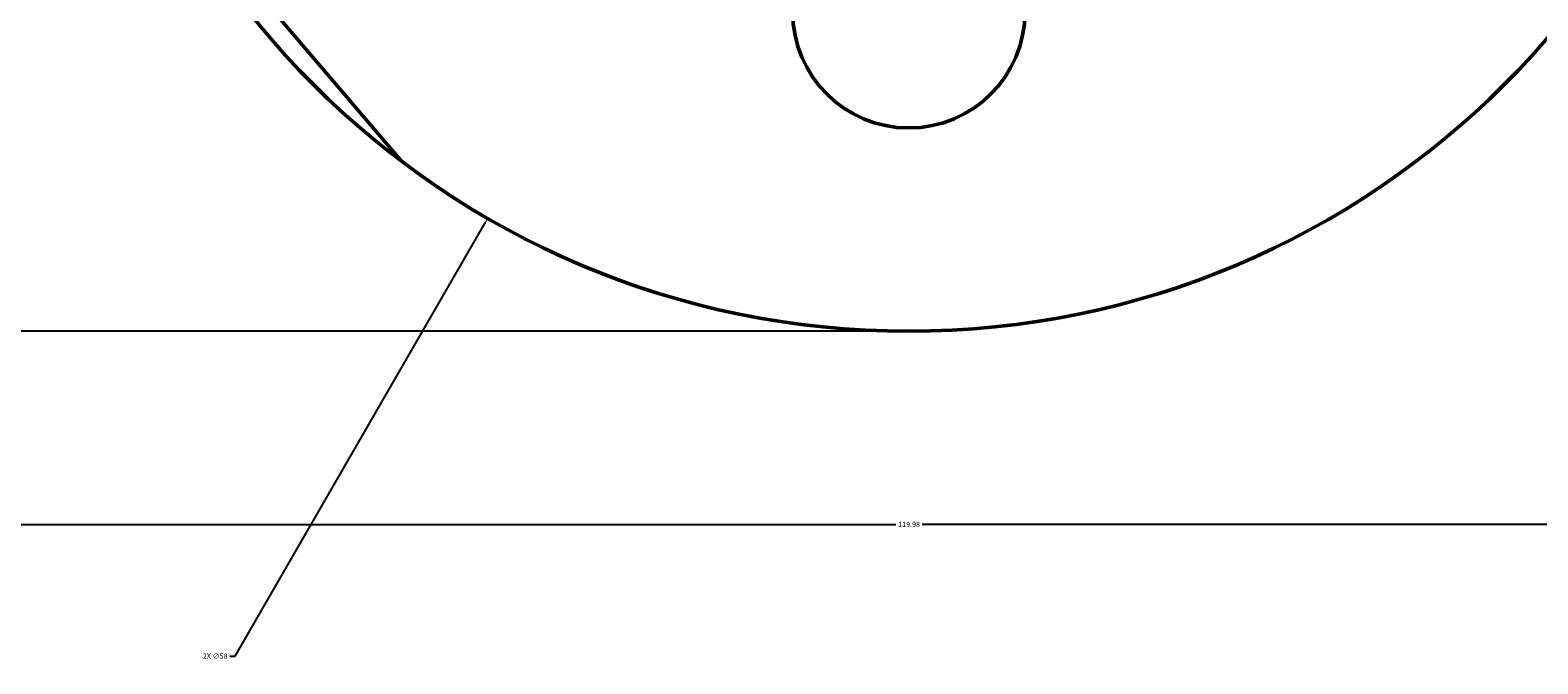
# Model space of a CAD drawing. Units: inches. Extents: x -11 to 126, y -62 to 82.
# Tile 2 of 10: x 29 to 81, y -62 to -40. Entities that reach past the tile are written whole.
import ezdxf

# ---------------------------------------------------------------- set-up
doc = ezdxf.new("R2010")
doc.units = ezdxf.units.IN
doc.header["$MEASUREMENT"] = 0
doc.layers.add('M-DIMS', color=2, linetype='Continuous', lineweight=18)
doc.layers.add('M-OUTL', color=7, linetype='Continuous', lineweight=50)
doc.styles.get("Standard").update_dxf_attribs({"font": 'arial.ttf'})
doc.dimstyles.get("Standard").update_dxf_attribs({"dimtxt": 0.18, "dimasz": 0.18, "dimexe": 0.18, "dimexo": 0.0625, "dimgap": 0.09, "dimtad": 0, "dimtih": 1, "dimtoh": 1, "dimdec": 4, "dimzin": 0, "dimdsep": 46, "dimtxsty": 'Standard', "dimcen": 0.09, "dimadec": 0, "dimazin": 0, "dimtfac": 1, "dimtdec": 4, "dimtofl": 0, "dimtmove": 0, "dimatfit": 3, "dimfxl": 1, "dimtolj": 1, "dimtzin": 0, "dimarcsym": 0})

# ---------------------------------------------------------------- blocks, each defined once
blk = doc.blocks.new('*U3')
blk.add_circle((0, 0), 4)
blk = doc.blocks.new('*U4')
at = {"layer": 'M-OUTL', "color": 0, "linetype": 'ByBlock', "lineweight": -2, "transparency": 16777216}
blk.add_blockref('*U3', (59.232, -3.646), dxfattribs=at)
for p, rotation in [((43.643, -12.646), 59.99999999999999), ((74.82, -12.646), 300), ((43.643, -30.646), 120), ((74.82, -30.646), 240), ((59.232, -39.646), 180)]:
    blk.add_blockref('*U3', p, dxfattribs=dict(at, rotation=rotation))
blk = doc.blocks.new('*D5')
at = {"layer": 'Defpoints', "color": 0, "transparency": 16777216}
for p in [(119.232, 12.354), (-0.749, 11.479), (119.232, -57.296)]:
    blk.add_point(p, dxfattribs=at)
at = {"layer": 'M-DIMS', "color": 0, "lineweight": -2, "transparency": 16777216}
for p, q in [((119.232, 12.292), (119.232, -57.476)), ((-0.749, 11.416), (-0.749, -57.476)), ((-0.569, -57.296), (58.786, -57.296)), ((119.052, -57.296), (59.696, -57.296))]:
    blk.add_line(p, q, dxfattribs=at)
at = {"layer": 'M-DIMS', "color": 0, "transparency": 16777216}
for points in [[(-0.569, -57.266), (-0.569, -57.326), (-0.749, -57.296)], [(119.052, -57.266), (119.052, -57.326), (119.232, -57.296)]]:
    blk.add_solid(points, dxfattribs=at)
at = {"layer": 'M-DIMS', "color": 0, "transparency": 16777216, "insert": (59.241, -57.296), "char_height": 0.18, "attachment_point": 5}
blk.add_mtext('\\A1;119.98', dxfattribs=at)
blk = doc.blocks.new('*D6')
at = {"layer": 'Defpoints', "color": 0, "transparency": 16777216}
for p in [(-7.399, 75.354), (59.232, 75.354), (59.232, -50.646)]:
    blk.add_point(p, dxfattribs=at)
at = {"layer": 'M-DIMS', "color": 0, "lineweight": -2, "transparency": 16777216}
for p, q in [((59.169, 75.354), (-7.579, 75.354)), ((-7.399, 75.174), (-7.399, 12.536)), ((-7.399, -50.466), (-7.399, 12.172)), ((59.169, -50.646), (-7.579, -50.646))]:
    blk.add_line(p, q, dxfattribs=at)
at = {"layer": 'M-DIMS', "color": 0, "transparency": 16777216}
for points in [[(-7.429, 75.174), (-7.369, 75.174), (-7.399, 75.354)], [(-7.429, -50.466), (-7.369, -50.466), (-7.399, -50.646)]]:
    blk.add_solid(points, dxfattribs=at)
at = {"layer": 'M-DIMS', "color": 0, "transparency": 16777216, "insert": (-7.399, 12.354), "char_height": 0.18, "attachment_point": 5}
blk.add_mtext('\\A1;126', dxfattribs=at)
blk = doc.blocks.new('*D13')
at = {"layer": 'Defpoints', "color": 0, "transparency": 16777216}
for p in [(73.731, 3.469), (44.732, -46.761)]:
    blk.add_point(p, dxfattribs=at)
at = {"layer": 'M-DIMS', "color": 0, "lineweight": -2, "transparency": 16777216}
for p, q in [((59.142, -21.646), (59.322, -21.646)), ((59.232, -21.736), (59.232, -21.556)), ((36.032, -61.83), (44.642, -46.917)), ((35.852, -61.83), (36.032, -61.83))]:
    blk.add_line(p, q, dxfattribs=at)
at = {"layer": 'M-DIMS', "color": 0, "transparency": 16777216}
blk.add_solid([(44.616, -46.902), (44.668, -46.932), (44.732, -46.761)], dxfattribs=at)
at = {"layer": 'M-DIMS', "color": 0, "transparency": 16777216, "insert": (35.345, -61.83), "char_height": 0.18, "attachment_point": 5}
blk.add_mtext('\\A1;2X ∅58', dxfattribs=at)

msp = doc.modelspace()

# ---------------------------------------------------------------- linework, layer by layer
at = {"layer": 'M-OUTL'}
msp.add_line((3.002, 0.666), (41.77, -44.799), dxfattribs=at)
msp.add_circle((59.232, -21.646), 29, dxfattribs=at)

# ---------------------------------------------------------------- block references
msp.add_blockref('*U4', (0, 0), dxfattribs=at)

# ---------------------------------------------------------------- dimensions: what is measured, and where the dimension line sits
at = {"layer": 'M-DIMS'}
dim = msp.add_linear_dim(base=(-7.399, 75.354), p1=(59.232, -50.646), p2=(59.232, 75.354), angle=90, dimstyle='Standard', override={"dimdec": 0, "dimlfac": 1, "dimrnd": 0, "dimzin": 0, "dimdsep": 46, "dimlunit": 2}, dxfattribs=at)
dim.commit()
dim.dimension.update_dxf_attribs({"geometry": '*D6', "text_midpoint": (-7.399, 12.354)})
dim = msp.add_linear_dim(base=(119.232, -57.296), p1=(-0.749, 11.479), p2=(119.232, 12.354), dimstyle='Standard', override={"dimdec": 2, "dimlfac": 1, "dimrnd": 0, "dimzin": 0, "dimdsep": 46, "dimlunit": 2}, dxfattribs=at)
dim.commit()
dim.dimension.update_dxf_attribs({"geometry": '*D5', "text_midpoint": (59.241, -57.296)})
dim = msp.add_diameter_dim_2p(p1=(73.731, 3.469), p2=(44.732, -46.761), text='2X <>', dimstyle='Standard', override={"dimdec": 0, "dimlfac": 1, "dimrnd": 0, "dimzin": 0, "dimdsep": 46, "dimlunit": 2}, dxfattribs=at)
dim.commit()
dim.dimension.update_dxf_attribs({"geometry": '*D13', "text_midpoint": (35.345, -61.83), "dimtype": 163})

doc.saveas('drawing.dxf')
